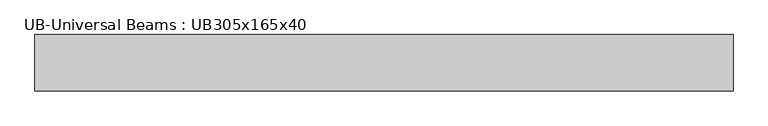
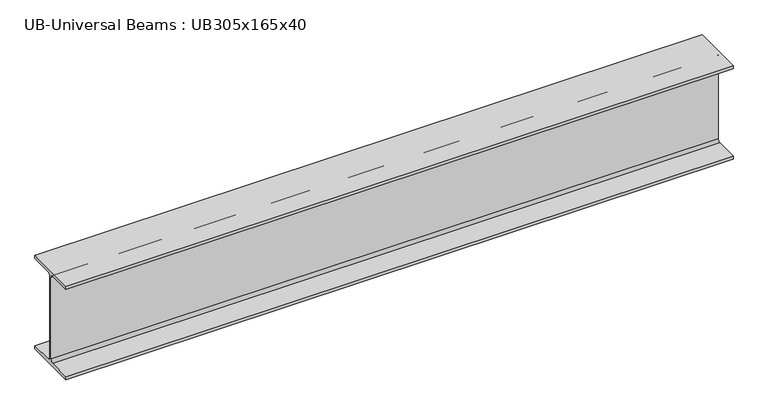
"""IFC4 building model written with IfcOpenShell, lengths in millimetres: beam geometry, UB-Universal Beams : UB305x165x40."""

from ifc_helpers import new_model, si_unit, point, frame, frame_2d, origin, place, context, project, spatial, polyline, circle_curve, trimmed, segment, composite_curve, outline, extrude, source, transform, mapped, element, save


def ub_universal_beams_ub305x165x40_ea68f55e(model_context):
    return source(origin(), model_context, "Body", "SweptSolid", [
        extrude(outline(composite_curve([segment(polyline([(82.5, -141.5), (82.5, -151.7), (-82.5, -151.7), (-82.5, -141.5), (-11.9, -141.5)]), True, "CONTINUOUS"), segment(trimmed(circle_curve(frame_2d((-11.9, -132.6)), 8.9), [point((-11.9, -141.5))], [point((-3.0, -132.6))], True, "CARTESIAN"), True, "CONTINUOUS"), segment(polyline([(-3.0, -132.6), (-3.0, 132.6)]), True, "CONTINUOUS"), segment(trimmed(circle_curve(frame_2d((-11.9, 132.6)), 8.9), [point((-3.0, 132.6))], [point((-11.9, 141.5))], True, "CARTESIAN"), True, "CONTINUOUS"), segment(polyline([(-11.9, 141.5), (-82.5, 141.5), (-82.5, 151.7), (82.5, 151.7), (82.5, 141.5), (11.9, 141.5)]), True, "CONTINUOUS"), segment(trimmed(circle_curve(frame_2d((11.9, 132.6)), 8.9), [point((11.9, 141.5))], [point((3.0, 132.6))], True, "CARTESIAN"), True, "CONTINUOUS"), segment(polyline([(3.0, 132.6), (3.0, -132.6)]), True, "CONTINUOUS"), segment(trimmed(circle_curve(frame_2d((11.9, -132.6)), 8.9), [point((3.0, -132.6))], [point((11.9, -141.5))], True, "CARTESIAN"), True, "CONTINUOUS"), segment(polyline([(11.9, -141.5), (82.5, -141.5)]), True, "CONTINUOUS")], self_intersect=False)), frame((-962.8, 0.0, 0.0), z_axis=(1.0, 0.0, 0.0), x_axis=(0.0, 1.0, 0.0)), (0.0, 0.0, 1.0), 2047.0),
    ])


if __name__ == "__main__":
    model = new_model("IFC4")
    model_context = context("Model", 3, world=origin())
    ifc_project = project(units=[si_unit("LENGTHUNIT", "METRE", prefix="MILLI")], contexts=[model_context])
    site = spatial("IfcSite", under=ifc_project)
    building = spatial("IfcBuilding", under=site)
    placement = place(None, origin())
    ub_universal_beams_ub305x165x40_shape = ub_universal_beams_ub305x165x40_ea68f55e(model_context)
    element("IfcBeam", 1, ObjectType="UB-Universal Beams : UB305x165x40", at=placement, inside=building, context=model_context, shape_type="MappedRepresentation", body=[
        mapped(ub_universal_beams_ub305x165x40_shape, transform((0.0, 0.0, 0.0), x_axis=(1.0, 0.0, 0.0), y_axis=(0.0, 1.0, 0.0), z_axis=(0.0, 0.0, 1.0))),
    ])
    save(model, "model.ifc")

# Revit data of these elements
# Type "UB-Universal Beams : UB305x165x40"
#   Section Name Key = "UB305X165X40"
#   Width = 16.5 cm
#   Web Thickness = 0.6 cm
#   Web Fillet = 0.89 cm
#   Warping Constant = 164000.0 cm⁶
#   Torsional Moment of Inertia = 14.70 cm⁴
#   Section Area = 51.3 cm²
#   Plastic Modulus weak axis = 142.0 cm³
#   Plastic Modulus strong axis = 623.0 cm³
#   Nominal Weight = 40.2999 kgf/m
#   Moment of Inertia weak axis = 764.00 cm⁴
#   Moment of Inertia strong axis = 8503.00 cm⁴
#   Height = 30.34 cm
#   Flange Thickness = 1.02 cm
#   Elastic Modulus weak axis = 92.6 cm³
#   Elastic Modulus strong axis = 560.0 cm³
#   Centroid Vertical = 15.17 cm
#   Centroid Horizontal = 8.25 cm
#   Bolt Spacing = 9.0 cm
#   Length [instance default] = 1500 mm
#   Structural Material [instance default] = Metal - Steel 43-275
#   Type Comments = ""
#   Assembly Code = ""
# Element 1 (IfcBeam, "UB-Universal Beams : UB305x165x40")
#   Materials on its faces: "Metal - Steel 43-275"
# Materials
#   "Metal - Steel 43-275": class "Metal", colour RGB 247 247 247, transparency 0, Cost = 0
